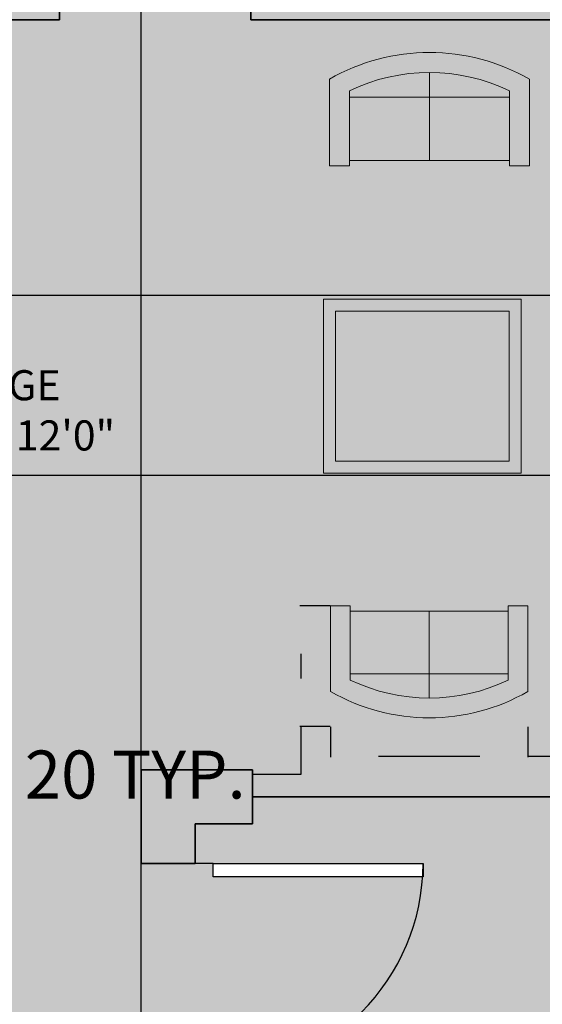
# Model space of a CAD drawing. Units: inches. Extents: x 389 to 971, y 148 to 870.
# Tile 12 of 14: x 670 to 757, y 428 to 592. Entities that reach past the tile are written whole.
import ezdxf

# ---------------------------------------------------------------- set-up
doc = ezdxf.new("R2010")
doc.units = ezdxf.units.IN
doc.header["$MEASUREMENT"] = 0
for name, color, linetype, lineweight in [('A-ANNO-DIMS', 2, 'Continuous', 18), ('A-AREA-IDEN', 7, 'Continuous', 18), ('A-DOOR', 4, 'Continuous', 25), ('A-FLOR-BASE-PATT', 8, 'Continuous', 13), ('A-FURN', 8, 'Continuous', 18), ('A-WALL', 7, 'Continuous', 35), ('L-GRND-BASE-PATT', 8, 'Continuous', 13)]:
    doc.layers.add(name, color=color, linetype=linetype, lineweight=lineweight)
for name, color, linetype, lineweight, true_color in [('A-FURN-SURF-PATT', 9, 'Continuous', 13, 0xd6bdce), ('A-WALL-PATT', 18, 'Continuous', 13, 0x000000), ('L-GRND-PATT', 39, 'Continuous', 13, 0x603913)]:
    doc.layers.add(name, color=color, linetype=linetype, lineweight=lineweight, true_color=true_color)
doc.styles.get("Standard").update_dxf_attribs({"font": 'arial.ttf'})
doc.dimstyles.get("Standard").update_dxf_attribs({"dimtxt": 8, "dimasz": 8, "dimexe": 0.18, "dimexo": 0.0625, "dimgap": 0.09, "dimtad": 0, "dimtih": 1, "dimtoh": 1, "dimdec": 0, "dimzin": 0, "dimdsep": 46, "dimlunit": 3, "dimtxsty": 'Standard', "dimcen": 0.09, "dimadec": 0, "dimazin": 0, "dimtfac": 1, "dimtdec": 0, "dimtofl": 0, "dimtmove": 0, "dimatfit": 3, "dimfxl": 1, "dimtolj": 1, "dimtzin": 0, "dimarcsym": 0})

# ---------------------------------------------------------------- blocks, each defined once
blk = doc.blocks.new('*U5')
for p, q in [((0, 0), (0, -6)), ((28, 0), (28, -6))]:
    blk.add_line(p, q)
blk.add_lwpolyline([(0, 0), (0, 28), (1.75, 28), (1.75, 0)], close=True)
blk.add_arc((0, 0), 28, 0, 90)
blk = doc.blocks.new('Sofa - Roundback Loveseat 5 ft.')
for p, q in [((0, -32.44198), (0, -5.99998)), ((-24, -33.99998), (-24, -11.46958)), ((24.00004, -33.99998), (24.00004, -11.46958)), ((-23.9998, -13.38178), (23.99986, -13.38178)), ((-24, -32.44198), (24.00004, -32.44198))]:
    blk.add_line(p, q)
for points in [[(-24, -33.99998), (-30, -33.99998), (-30, -7.99998)], [(30.00004, -7.99998), (30.00004, -33.99998), (24.00004, -33.99998)]]:
    blk.add_lwpolyline(points)
for centre, radius, start, end in [((0, -60.24998), 60.24998, 60.13715, 119.8628), ((0, -61.38438), 55.38444, 64.32083, 115.6792)]:
    blk.add_arc(centre, radius, start, end)
blk = doc.blocks.new('COFFEE-TABLE-RECT')
for points in [[(0, 28.98), (32.94, 28.98), (32.94, 0), (0, 0)], [(2, 26.98), (30.94, 26.98), (30.94, 2), (2, 2)]]:
    blk.add_lwpolyline(points, close=True)
blk = doc.blocks.new('*D40')
at = {"layer": 'A-ANNO-DIMS', "color": 0, "lineweight": -2, "transparency": 16777216}
for p, q in [((721.8, 473.76), (721.8, 468.71)), ((754.7, 473.76), (754.7, 468.71)), ((729.8, 468.89), (746.7, 468.89)), ((754.7, 468.89), (762.7, 468.89))]:
    blk.add_line(p, q, dxfattribs=at)
at = {"layer": 'A-ANNO-DIMS', "color": 0, "transparency": 16777216}
for points in [[(729.8, 470.23), (729.8, 467.56), (721.8, 468.89)], [(746.7, 470.23), (746.7, 467.56), (754.7, 468.89)]]:
    blk.add_solid(points, dxfattribs=at)
at = {"layer": 'Defpoints', "color": 0, "transparency": 16777216}
for p in [(721.8, 473.83), (754.7, 473.83), (754.7, 468.89)]:
    blk.add_point(p, dxfattribs=at)
at = {"layer": 'A-ANNO-DIMS', "color": 0, "transparency": 16777216, "insert": (813.14, 468.89), "char_height": 8, "attachment_point": 5}
blk.add_mtext('\\A1;LOVESEAT 33 TYP.', dxfattribs=at)
blk = doc.blocks.new('*D41')
at = {"layer": 'A-ANNO-DIMS', "color": 0, "lineweight": -2, "transparency": 16777216}
for p, q in [((721.74, 493.93), (716.69, 493.93)), ((716.87, 485.93), (716.87, 481.83)), ((721.74, 473.83), (716.69, 473.83)), ((716.87, 473.83), (716.87, 465.83)), ((716.87, 465.83), (708.87, 465.83))]:
    blk.add_line(p, q, dxfattribs=at)
at = {"layer": 'A-ANNO-DIMS', "color": 0, "transparency": 16777216}
for points in [[(715.53, 485.93), (718.2, 485.93), (716.87, 493.93)], [(715.53, 481.83), (718.2, 481.83), (716.87, 473.83)]]:
    blk.add_solid(points, dxfattribs=at)
at = {"layer": 'Defpoints', "color": 0, "transparency": 16777216}
for p in [(721.8, 493.93), (716.87, 473.83), (721.8, 473.83)]:
    blk.add_point(p, dxfattribs=at)
at = {"layer": 'A-ANNO-DIMS', "color": 0, "transparency": 16777216, "insert": (689.24, 465.83), "char_height": 8, "attachment_point": 5}
blk.add_mtext('\\A1;20 TYP.', dxfattribs=at)
blk = doc.blocks.new('*D48')
at = {"layer": 'A-ANNO-DIMS', "color": 0, "lineweight": -2, "transparency": 16777216}
for p, q in [((595.45, 545.73), (878.72, 545.73)), ((878.54, 537.73), (878.54, 534.91)), ((878.54, 523.73), (878.54, 526.55)), ((595.45, 515.73), (878.72, 515.73))]:
    blk.add_line(p, q, dxfattribs=at)
at = {"layer": 'A-ANNO-DIMS', "color": 0, "transparency": 16777216}
for points in [[(877.21, 537.73), (879.87, 537.73), (878.54, 545.73)], [(877.21, 523.73), (879.87, 523.73), (878.54, 515.73)]]:
    blk.add_solid(points, dxfattribs=at)
at = {"layer": 'Defpoints', "color": 0, "transparency": 16777216}
for p in [(595.39, 545.73), (878.54, 545.73), (595.39, 515.73)]:
    blk.add_point(p, dxfattribs=at)
at = {"layer": 'A-ANNO-DIMS', "color": 0, "transparency": 16777216, "insert": (878.54, 530.73), "char_height": 8, "attachment_point": 5}
blk.add_mtext('\\A1;30.005', dxfattribs=at)
blk = doc.blocks.new('*D52')
at = {"layer": 'A-ANNO-DIMS', "color": 0, "lineweight": -2, "transparency": 16777216}
for p, q in [((640.06, 864.97), (632.06, 864.97)), ((648.06, 388.98), (648.06, 865.15)), ((690.22, 388.98), (690.22, 865.15)), ((698.22, 864.97), (706.22, 864.97))]:
    blk.add_line(p, q, dxfattribs=at)
at = {"layer": 'A-ANNO-DIMS', "color": 0, "transparency": 16777216}
for points in [[(640.06, 866.3), (640.06, 863.64), (648.06, 864.97)], [(698.22, 866.3), (698.22, 863.64), (690.22, 864.97)]]:
    blk.add_solid(points, dxfattribs=at)
at = {"layer": 'Defpoints', "color": 0, "transparency": 16777216}
for p in [(690.22, 864.97), (648.06, 388.92), (690.22, 388.92)]:
    blk.add_point(p, dxfattribs=at)
at = {"layer": 'A-ANNO-DIMS', "color": 0, "transparency": 16777216, "insert": (669.14, 864.97), "char_height": 8, "attachment_point": 5}
blk.add_mtext('\\A1;42.155', dxfattribs=at)

msp = doc.modelspace()

# ---------------------------------------------------------------- hatches: boundary and pattern name
at = {"layer": 'A-FLOR-BASE-PATT'}
h = msp.add_hatch(color=256, dxfattribs=at)
h.dxf.hatch_style = 1
h.paths.add_polyline_path([(634.6594, 428.4021), (634.6594, 427.0792), (634.6305, 427.0792, -0.40145271), (604.4225, 398.1652), (604.0817, 398.1199, -0.40145271), (632.0195, 371.3788), (632.0462, 371.3788), (632.0462, 370.1554), (604.387, 370.1554), (604.387, 366.7191), (640.0296, 366.7191), (640.0296, 321.4969, 1), (647.061, 321.4969), (647.061, 412.9189), (690.216, 412.9189), (690.216, 416.0006), (694.716, 416.0006), (702.2145, 416.0006, 0.39601219), (737.1392, 448.8066), (702.2145, 448.8066), (702.2145, 450.9936), (694.716, 450.9936), (690.216, 450.9936), (690.216, 466.6012), (708.7881, 466.6012), (708.7881, 462.1012), (784.6145, 462.1012), (784.6145, 466.6012), (794.216, 466.6012), (794.216, 591.6445), (708.5171, 591.6445), (708.5171, 596.1445), (708.5171, 602.9755, 0.39601219), (678.6314, 634.7912), (678.6314, 602.9755), (676.6391, 602.9755), (676.6391, 596.1445), (676.6391, 591.6445), (661.216, 591.6445), (661.216, 632.6445), (653.109, 632.6445), (653.109, 641.6445), (653.109, 642.1751), (651.6417, 642.1751), (651.6417, 675.6801, 0.40145271), (619.5719, 642.1751), (619.5719, 637.1445), (619.5147, 632.6445), (604.387, 632.6445), (604.387, 545.7317), (595.3894, 545.7317), (595.3894, 544.4199), (565.4338, 544.4199, 0.40145271), (595.3894, 515.7475), (599.887, 515.7475), (604.387, 515.7271), (604.387, 428.4021)])
h.paths.add_polyline_path([(721.8003, 493.9292), (725.0899, 493.9292), (725.0899, 493.075), (751.4065, 493.075), (751.4065, 493.9292), (754.6961, 493.9292), (754.6961, 479.6744, -0.26666697), (721.8003, 479.6744)], flags=16)
h.paths.add_polyline_path([(720.6421, 516.0583), (720.6421, 545.0393), (753.5806, 545.0393), (753.5806, 516.0583)], flags=16)
h.paths.add_polyline_path([(722.6421, 518.0583), (722.6421, 543.0393), (751.5806, 543.0393), (751.5806, 518.0583)], flags=0)
h.paths.add_polyline_path([(763.7396, 488.5801), (763.7822, 488.1156), (764.1436, 488.1761)], flags=16)
h.paths.add_polyline_path([(777.9011, 479.7417), (778.0475, 480.1886), (777.4745, 480.275)], flags=16)
h.paths.add_polyline_path([(762.3329, 503.5919), (762.3329, 507.1718), (763.2624, 507.1718), (763.2624, 550.1306), (762.3329, 550.1306), (762.3329, 553.7105), (777.8458, 553.7105, -0.19047621), (777.8458, 503.5919)], flags=16)
h.paths.add_polyline_path([(721.6097, 567.2898), (721.6097, 581.7362, -0.26666697), (754.9475, 581.7362), (754.9475, 567.2898), (751.6137, 567.2898), (751.6137, 568.1555), (724.9435, 568.1555), (724.9435, 567.2898)], flags=16)
h.paths.add_polyline_path([(774.6347, 521.4914), (774.6347, 535.811), (778.6837, 535.811, -0.04962821), (778.6837, 521.4914)], flags=0)
h.paths.add_polyline_path([(764.6624, 576.8996), (764.7454, 576.4742), (765.0717, 576.4903)], flags=16)
h.paths.add_polyline_path([(777.2772, 570.3652), (777.4444, 570.8756), (776.7899, 570.9743)], flags=16)
h.paths.add_polyline_path([(644.2892, 516.9956), (685.2491, 516.9956), (685.2491, 535.7223), (644.2892, 535.7223)], flags=24)
h = msp.add_hatch(color=256, dxfattribs=at)
h.dxf.hatch_style = 1
h.paths.add_polyline_path([(699.216, 294.6445), (733.8057, 294.6445), (810.0514, 294.6445), (839.216, 294.6445), (839.216, 457.6012), (784.6145, 457.6012), (784.6145, 462.1012), (708.7881, 462.1012), (708.7881, 457.6012), (699.216, 457.6012), (699.216, 450.9936), (702.2145, 450.9936), (737.2076, 450.9936), (737.2076, 448.8066), (737.1392, 448.8066, -0.39601219), (702.2145, 416.0006), (699.216, 416.0006)])
h.paths.add_polyline_path([(755.1859, 373.9163), (788.1244, 373.9163), (788.1244, 344.9352), (755.1859, 344.9352)], flags=16)
h.paths.add_polyline_path([(757.1859, 371.9163), (786.1244, 371.9163), (786.1244, 346.9352), (757.1859, 346.9352)], flags=0)
h.paths.add_polyline_path([(746.1376, 327.3223), (750.14, 327.3223), (750.14, 326.2831), (798.1694, 326.2831), (798.1694, 327.3223), (802.1718, 327.3223), (802.1718, 309.9784, -0.19047621), (746.1376, 309.9784)], flags=16)
h.paths.add_polyline_path([(782.1596, 313.5685), (782.1596, 309.0415, -0.04962821), (766.1498, 309.0415), (766.1498, 313.5685)], flags=0)
h.paths.add_polyline_path([(804.6838, 390.5197), (803.6446, 390.5197), (803.6446, 394.5221), (820.9885, 394.5221, -0.19047621), (820.9885, 338.4879), (803.6446, 338.4879), (803.6446, 342.4903), (804.6838, 342.4903)], flags=16)
h.paths.add_polyline_path([(817.3984, 358.5001), (817.3984, 374.5099), (821.9254, 374.5099, -0.04962821), (821.9254, 358.5001)], flags=0)
h.paths.add_polyline_path([(806.8707, 326.6963), (806.4254, 327.1416), (806.4724, 326.6297)], flags=16)
h.paths.add_polyline_path([(822.0328, 317.4008), (822.1942, 317.8933), (821.5626, 317.9885)], flags=16)
h.paths.add_polyline_path([(808.1446, 418.9737), (808.2247, 418.5632), (808.5395, 418.5787)], flags=16)
h.paths.add_polyline_path([(820.3159, 412.669), (820.4772, 413.1615), (819.8457, 413.2568)], flags=16)
h.paths.add_polyline_path([(750.6082, 393.6667), (791.5681, 393.6667), (791.5681, 412.3933), (750.6082, 412.3933)], flags=24)
at = {"layer": 'A-FURN-SURF-PATT'}
h = msp.add_hatch(color=256, dxfattribs=at)
h.dxf.hatch_style = 1
h.paths.add_polyline_path([(754.9475, 581.7362, 0.26666697), (721.6097, 581.7362), (721.6097, 567.2898), (724.9435, 567.2898), (724.9435, 579.8081, -0.22792319), (751.6137, 579.8081), (751.6137, 567.2898), (754.9475, 567.2898)])
h = msp.add_hatch(color=256, dxfattribs=at)
h.dxf.hatch_style = 1
h.paths.add_polyline_path([(738.2786, 578.7459), (738.2786, 582.8475, 0.11251869), (724.9435, 579.8081), (724.9435, 578.7459)])
h = msp.add_hatch(color=256, dxfattribs=at)
h.dxf.hatch_style = 1
h.paths.add_polyline_path([(751.6137, 578.7459), (751.6137, 579.8081, 0.11251889), (738.2786, 582.8475), (738.2786, 578.7459)])
h = msp.add_hatch(color=256, dxfattribs=at)
h.dxf.hatch_style = 1
h.paths.add_polyline_path([(738.2786, 568.1555), (738.2786, 578.7459), (724.9435, 578.7459), (724.9435, 568.1555)])
h = msp.add_hatch(color=256, dxfattribs=at)
h.dxf.hatch_style = 1
h.paths.add_polyline_path([(751.6137, 568.1555), (751.6137, 578.7459), (738.2786, 578.7459), (738.2786, 568.1555)])
h = msp.add_hatch(color=256, dxfattribs=at)
h.dxf.hatch_style = 1
h.paths.add_polyline_path([(720.6421, 545.0393), (720.6421, 516.0583), (753.5806, 516.0583), (753.5806, 545.0393)])
h.paths.add_polyline_path([(751.5806, 543.0393), (751.5806, 518.0583), (722.6421, 518.0583), (722.6421, 543.0393)], flags=16)
h = msp.add_hatch(color=256, dxfattribs=at)
h.dxf.hatch_style = 1
h.paths.add_polyline_path([(751.5806, 518.0583), (751.5806, 543.0393), (722.6421, 543.0393), (722.6421, 518.0583)])
h = msp.add_hatch(color=256, dxfattribs=at)
h.dxf.hatch_style = 1
h.paths.add_polyline_path([(721.8003, 479.6744, 0.26666697), (754.6961, 479.6744), (754.6961, 493.9292), (751.4065, 493.9292), (751.4065, 481.5769, -0.22792319), (725.0899, 481.5769), (725.0899, 493.9292), (721.8003, 493.9292)])
h = msp.add_hatch(color=256, dxfattribs=at)
h.dxf.hatch_style = 1
h.paths.add_polyline_path([(738.2482, 493.075), (725.0899, 493.075), (725.0899, 482.625), (738.2482, 482.625)])
h = msp.add_hatch(color=256, dxfattribs=at)
h.dxf.hatch_style = 1
h.paths.add_polyline_path([(751.4065, 482.625), (751.4065, 493.075), (738.2482, 493.075), (738.2482, 482.625)])
h = msp.add_hatch(color=256, dxfattribs=at)
h.dxf.hatch_style = 1
h.paths.add_polyline_path([(738.2482, 482.625), (725.0899, 482.625), (725.0899, 481.5769, 0.11251869), (738.2482, 478.5778)])
h = msp.add_hatch(color=256, dxfattribs=at)
h.dxf.hatch_style = 1
h.paths.add_polyline_path([(751.4065, 481.5769), (751.4065, 482.625), (738.2482, 482.625), (738.2482, 478.5778, 0.11251889)])
at = {"layer": 'A-WALL-PATT'}
h = msp.add_hatch(color=256, dxfattribs=at)
h.dxf.hatch_style = 1
h.paths.add_polyline_path([(432.216, 434.6445), (436.3673, 434.6445), (436.3673, 443.6445), (432.216, 443.6445), (432.216, 830.6445), (746.216, 830.6445), (746.216, 823.8175), (755.216, 823.8175), (755.216, 825.6445), (839.216, 825.6445), (839.216, 803.5176), (839.216, 741.6445), (755.216, 741.6445), (755.216, 748.4596), (755.1859, 748.4596), (750.716, 748.4596), (746.216, 748.4596), (746.216, 732.6445), (839.216, 732.6445), (839.216, 600.6445), (708.5171, 600.6445), (708.5171, 596.1445), (708.5171, 591.6445), (794.216, 591.6445), (794.216, 587.4291), (803.216, 587.4291), (803.216, 591.6445), (839.216, 591.6445), (839.216, 466.6012), (803.216, 466.6012), (803.216, 471.0309), (794.216, 471.0309), (794.216, 466.6012), (784.6145, 466.6012), (784.6145, 457.6012), (839.216, 457.6012), (839.216, 447.6445), (839.216, 294.6445), (810.0514, 294.6445), (810.0514, 285.6445), (839.216, 285.6445), (839.216, 238.6445), (590.216, 238.6445), (590.216, 234.6445), (848.216, 234.6445), (848.216, 834.6445), (428.216, 834.6445), (428.216, 234.6445), (437.216, 234.6445), (437.216, 243.6445), (432.216, 243.6445)])
h = msp.add_hatch(color=256, dxfattribs=at)
h.dxf.hatch_style = 1
h.paths.add_polyline_path([(661.216, 785.6445), (661.216, 641.6445), (653.109, 641.6445), (653.109, 637.1445), (653.109, 632.6445), (661.216, 632.6445), (661.216, 591.6445), (676.6391, 591.6445), (676.6391, 600.6445), (670.216, 600.6445), (670.216, 785.6445), (685.2392, 785.6445), (685.2392, 794.6445), (662.4125, 794.6445), (606.2724, 794.6445), (606.2724, 785.6445), (616.7487, 785.6445)])
h = msp.add_hatch(color=256, dxfattribs=at)
h.dxf.hatch_style = 1
h.paths.add_polyline_path([(690.216, 466.6012), (690.216, 450.9936), (699.216, 450.9936), (699.216, 457.6012), (708.7881, 457.6012), (708.7881, 466.6012)])
at = {"layer": 'L-GRND-BASE-PATT'}
h = msp.add_hatch(color=256, dxfattribs=at)
h.dxf.hatch_style = 1
edge = h.paths.add_edge_path(flags=16)
edge.add_ellipse((8782.0026, 354.2473), major_axis=(-8296.9493, 0), ratio=0.84230387, start_angle=-0.09022909, end_angle=0.38386678, ccw=False)
edge.add_ellipse((485.0533, 368.2895), major_axis=(-1.1591, 0), ratio=0.84230387, start_angle=0, end_angle=90, ccw=False)
edge.add_line((483.8943, 368.2895), (483.8943, 387.6039))
edge.add_ellipse((485.0533, 387.2466), major_axis=(1.1591, 0), ratio=0.84230387, start_angle=90, end_angle=180, ccw=False)
edge.add_line((485.0533, 388.2229), (485.5047, 388.2229))
edge.add_ellipse((898.8202, 372.4897), major_axis=(413.7374, 0), ratio=0.84230387, start_angle=176.349572, end_angle=177.82005, ccw=False)
edge.add_ellipse((535.9119, 196.3855), major_axis=(-245.3972, 0), ratio=0.84230387, start_angle=-77.874034, end_angle=-76.219471, ccw=False)
edge.add_ellipse((535.9119, 201.7547), major_axis=(239.1274, 0), ratio=0.84230387, start_angle=100.209539, end_angle=102.444627, ccw=False)
edge.add_ellipse((473.3139, 564.9222), major_axis=(196.5637, 0), ratio=0.84230387, start_angle=-80.743434, end_angle=-77.445067)
edge.add_line((509.5535, 402.1941), (514.3535, 404.8483))
edge.add_line((514.3535, 404.8483), (514.3535, 404.7972))
edge.add_ellipse((514.3535, 404.2644), major_axis=(0.5795, 0), ratio=0.84230387, start_angle=52.06687, end_angle=90, ccw=False)
edge.add_line((514.6716, 404.6725), (519.1535, 402.1941))
edge.add_ellipse((555.3932, 564.9222), major_axis=(-196.5637, 0), ratio=0.84230387, start_angle=77.445067, end_angle=80.743434)
edge.add_ellipse((492.7951, 201.7547), major_axis=(239.1274, 0), ratio=0.84230387, start_angle=77.555373, end_angle=79.790461, ccw=False)
edge.add_ellipse((492.7951, 196.3855), major_axis=(245.3972, 0), ratio=0.84230387, start_angle=76.219471, end_angle=77.874034, ccw=False)
edge.add_ellipse((129.8868, 372.4897), major_axis=(-413.7374, 0), ratio=0.84230387, start_angle=182.17995, end_angle=183.650428, ccw=False)
edge.add_line((543.2023, 388.2229), (544.0779, 388.2229))
edge.add_ellipse((543.6537, 387.2466), major_axis=(-1.1591, 0), ratio=0.84230387, start_angle=180, end_angle=270, ccw=False)
edge.add_line((544.8128, 387.2466), (544.8128, 367.9322))
edge.add_ellipse((543.6537, 368.2895), major_axis=(1.1591, 0), ratio=0.84230387, start_angle=270, end_angle=360, ccw=False)
edge.add_ellipse((-7753.2956, 354.2473), major_axis=(-8296.9493, 0), ratio=0.84230387, start_angle=179.61613322, end_angle=180.09022909, ccw=False)
edge.add_line((543.3912, 298.6608), (544.0779, 298.6608))
edge.add_ellipse((543.6537, 297.6845), major_axis=(1.1591, 0), ratio=0.84230387, start_angle=0, end_angle=90, ccw=False)
edge.add_line((544.8128, 297.6845), (544.8128, 278.3701))
edge.add_ellipse((543.6537, 278.7275), major_axis=(-1.1591, 0), ratio=0.84230387, start_angle=90, end_angle=180, ccw=False)
edge.add_line((543.6537, 277.7512), (543.1566, 277.7512))
edge.add_ellipse((-7753.2956, 354.2473), major_axis=(-8296.9493, 0), ratio=0.84230387, start_angle=179.3813568, end_angle=179.47172853, ccw=False)
edge.add_ellipse((542.4236, 263.2763), major_axis=(-1.7386, 0), ratio=0.84230387, start_angle=179.371763, end_angle=248.464757, ccw=False)
edge.add_ellipse((-7753.8751, 354.2473), major_axis=(-8298.7403, 0), ratio=0.842303866, start_angle=179.35344592, end_angle=179.3717628, ccw=False)
edge.add_ellipse((540.0116, 260.6509), major_axis=(-4.1092, 0), ratio=0.84230387, start_angle=90, end_angle=179.353446, ccw=False)
edge.add_line((540.0116, 257.1897), (488.6954, 257.1897))
edge.add_ellipse((488.6954, 260.6509), major_axis=(4.1092, 0), ratio=0.84230387, start_angle=180.646554, end_angle=270, ccw=False)
edge.add_ellipse((8782.5821, 354.2473), major_axis=(-8298.7403, 0), ratio=0.842303872, start_angle=0.62823723, end_angle=0.64655411, ccw=False)
edge.add_ellipse((486.2834, 263.2763), major_axis=(-1.7386, 0), ratio=0.84230387, start_angle=-68.464756, end_angle=0.628237, ccw=False)
edge.add_ellipse((8782.0026, 354.2473), major_axis=(-8296.9493, 0), ratio=0.84230387, start_angle=0.52827147, end_angle=0.6465541, ccw=False)
edge.add_line((485.5504, 277.7512), (484.6291, 277.7512))
edge.add_ellipse((485.0533, 278.7275), major_axis=(-1.1591, 0), ratio=0.84230387, start_angle=0, end_angle=90, ccw=False)
edge.add_line((483.8943, 278.7275), (483.8943, 298.0418))
edge.add_ellipse((485.0533, 297.6845), major_axis=(1.1591, 0), ratio=0.84230387, start_angle=90, end_angle=180, ccw=False)
edge = h.paths.add_edge_path(flags=0)
edge.add_ellipse((8782.0026, 354.2473), major_axis=(-8295.7902, 0), ratio=0.84230387, start_angle=0.05559431, end_angle=0.37776419, ccw=False)
edge.add_line((486.2179, 346.1978), (489.3905, 335.8384))
edge.add_ellipse((3386.0114, 329.7263), major_axis=(-2896.63, 0), ratio=0.84230387, start_angle=-0.1208974, end_angle=0.3640763)
edge.add_line((489.4638, 311.3204), (486.4666, 299.5521))
edge = h.paths.add_edge_path(flags=0)
edge.add_ellipse((514.3535, 391.3731), major_axis=(-115.1513, 0), ratio=0.84230387, start_angle=76.401865, end_angle=103.598135)
edge.add_line((537.3428, 296.3333), (537.3428, 281.5897))
edge.add_ellipse((514.3535, 376.6295), major_axis=(-115.1513, 0), ratio=0.84230387, start_angle=76.401865, end_angle=103.598135, ccw=False)
edge.add_line((491.3643, 281.5897), (491.3643, 296.3333))
edge = h.paths.add_edge_path(flags=0)
edge.add_line((491.3643, 337.0752), (489.653, 349.9016))
edge.add_ellipse((510.1338, 298.7862), major_axis=(64.0481, 0), ratio=0.84230387, start_angle=94.277421, end_angle=111.834954, ccw=False)
edge.add_line((506.1068, 352.6274), (522.6002, 352.6274))
edge.add_ellipse((518.5732, 298.7862), major_axis=(64.0481, 0), ratio=0.84230387, start_angle=68.165046, end_angle=85.722579, ccw=False)
edge.add_line((539.0541, 349.9016), (537.3428, 337.0752))
edge.add_ellipse((516.5462, 287.5825), major_axis=(62.3305, 0), ratio=0.84230387, start_angle=67.208085, end_angle=85.12993)
edge.add_line((521.008, 339.949), (507.699, 339.949))
edge.add_ellipse((512.1609, 287.5825), major_axis=(62.3305, 0), ratio=0.84230387, start_angle=94.87007, end_angle=112.791915)
edge = h.paths.add_edge_path(flags=0)
edge.add_ellipse((493.6824, 273.9439), major_axis=(-2.3182, 0), ratio=0.84230387, start_angle=-90, end_angle=0, ccw=False)
edge.add_line((493.6824, 275.8965), (535.3743, 275.8965))
edge.add_ellipse((535.0246, 273.9439), major_axis=(2.3182, 0), ratio=0.84230387, start_angle=0, end_angle=90, ccw=False)
edge.add_line((537.3428, 273.9439), (537.3428, 258.6983))
edge.add_line((537.3428, 258.6983), (540.5912, 258.6983))
edge.add_ellipse((540.5912, 260.6509), major_axis=(-2.3182, 0), ratio=0.84230387, start_angle=90, end_angle=179.353446)
edge.add_line((540.5912, 258.6983), (487.7691, 258.6983))
edge.add_ellipse((488.1158, 260.6509), major_axis=(2.3182, 0), ratio=0.84230387, start_angle=180.646554, end_angle=270)
edge.add_line((488.1158, 258.6983), (491.3643, 258.6983))
edge.add_line((491.3643, 258.6983), (491.3643, 274.2384))
h.paths.add_polyline_path([(746.1376, 327.3223), (750.14, 327.3223), (750.14, 326.2831), (798.1694, 326.2831), (798.1694, 327.3223), (802.1718, 327.3223), (802.1718, 309.9784, -0.19047621), (746.1376, 309.9784)], flags=16)
h.paths.add_polyline_path([(782.1596, 313.5685), (782.1596, 309.0415, -0.04962821), (766.1498, 309.0415), (766.1498, 313.5685)], flags=0)
h.paths.add_polyline_path([(755.1859, 344.9352), (755.1859, 373.9163), (788.1244, 373.9163), (788.1244, 344.9352)], flags=16)
h.paths.add_polyline_path([(757.1859, 346.9352), (757.1859, 371.9163), (786.1244, 371.9163), (786.1244, 346.9352)], flags=0)
h.paths.add_polyline_path([(803.6446, 338.4879), (803.6446, 342.4903), (804.6838, 342.4903), (804.6838, 390.5197), (803.6446, 390.5197), (803.6446, 394.5221), (820.9885, 394.5221, -0.19047621), (820.9885, 338.4879)], flags=16)
h.paths.add_polyline_path([(806.8707, 326.6963), (806.4254, 327.1416), (806.4724, 326.6297)], flags=16)
h.paths.add_polyline_path([(822.0328, 317.4008), (822.1942, 317.8933), (821.5626, 317.9885)], flags=16)
h.paths.add_polyline_path([(817.3984, 358.5001), (817.3984, 374.5099), (821.9254, 374.5099, -0.04962821), (821.9254, 358.5001)], flags=0)
h.paths.add_polyline_path([(808.1446, 418.9737), (808.2247, 418.5632), (808.5395, 418.5787)], flags=16)
h.paths.add_polyline_path([(820.3159, 412.669), (820.4772, 413.1615), (819.8457, 413.2568)], flags=16)
h.paths.add_polyline_path([(466.3155, 235.5246), (517.3807, 235.5246), (517.3807, 244.4269), (466.3155, 244.4269)], flags=24)
h.paths.add_polyline_path([(739.8737, 256.2), (815.404, 256.2), (815.404, 265.3454), (739.8737, 265.3454)], flags=24)
h.paths.add_polyline_path([(750.6082, 393.6667), (791.5681, 393.6667), (791.5681, 412.3933), (750.6082, 412.3933)], flags=24)
h.paths.add_polyline_path([(438.9631, 410.0619), (484.6204, 410.0619), (484.6204, 429.1217), (438.9631, 429.1217)], flags=24)
edge = h.paths.add_edge_path()
edge.add_line((839.216, 285.6445), (611.8787, 285.6445))
edge.add_line((611.8787, 285.6445), (604.387, 285.6445))
edge.add_line((604.387, 285.6445), (595.387, 285.6445))
edge.add_line((595.387, 285.6445), (595.387, 370.1554))
edge.add_line((595.387, 370.1554), (604.0817, 370.1554))
edge.add_line((604.0817, 370.1554), (604.0817, 371.3788))
edge.add_line((604.0817, 371.3788), (632.0195, 371.3788))
edge.add_arc((604.0817, 370.1554), 27.9645, 2.507491, 90)
edge.add_line((604.0817, 398.1199), (599.887, 398.1652))
edge.add_line((599.887, 398.1652), (604.4225, 398.1652))
edge.add_arc((604.4225, 428.4021), 30.2369, 270, 357.492509)
edge.add_line((634.6305, 427.0792), (604.4225, 427.0792))
edge.add_line((604.4225, 427.0792), (604.4225, 428.4021))
edge.add_line((604.4225, 428.4021), (599.887, 428.4021))
edge.add_line((599.887, 428.4021), (595.387, 428.4021))
edge.add_line((595.387, 428.4021), (595.387, 434.6445))
edge.add_line((595.387, 434.6445), (585.0791, 434.6445))
edge.add_line((585.0791, 434.6445), (540.3922, 434.6445))
edge.add_line((540.3922, 434.6445), (526.7125, 434.6445))
edge.add_line((526.7125, 434.6445), (488.4095, 434.6445))
edge.add_line((488.4095, 434.6445), (432.216, 434.6445))
edge.add_line((432.216, 434.6445), (432.216, 243.6445))
edge.add_line((432.216, 243.6445), (437.216, 243.6445))
edge.add_line((437.216, 243.6445), (437.216, 234.6445))
edge.add_line((437.216, 234.6445), (581.216, 234.6445))
edge.add_line((581.216, 234.6445), (581.216, 238.6445))
edge.add_line((581.216, 238.6445), (581.216, 243.6445))
edge.add_line((581.216, 243.6445), (590.216, 243.6445))
edge.add_line((590.216, 243.6445), (590.216, 238.6445))
edge.add_line((590.216, 238.6445), (839.216, 238.6445))
edge.add_line((839.216, 238.6445), (839.216, 285.6445))
at = {"layer": 'L-GRND-PATT'}
h = msp.add_hatch(dxfattribs=at)
h.set_pattern_fill('EARTH', color=256, angle=45)
h.set_pattern_definition([(45, (0, 0), (0, 8.980256), [6.35, -6.35]), (45, (-1.684, 1.684), (0, 8.980256), [6.35, -6.35]), (45, (-3.3676, 3.3676), (0, 8.980256), [6.35, -6.35]), (135, (-3.3676, 4.49), (-8.980256, 0), [6.35, -6.35]), (135, (-1.684, 6.174), (-8.980256, 0), [6.35, -6.35]), (135, (0, 7.858), (-8.980256, 0), [6.35, -6.35])])
h.paths.add_polyline_path([(432.216, 243.6445), (437.216, 243.6445), (437.216, 234.6445), (581.216, 234.6445), (581.216, 238.6445), (581.216, 243.6445), (590.216, 243.6445), (590.216, 238.6445), (839.216, 238.6445), (839.216, 285.6445), (810.0514, 285.6445), (733.8057, 285.6445), (684.2434, 285.6445), (611.8787, 285.6445), (604.387, 285.6445), (595.387, 285.6445), (595.387, 370.1554), (604.0817, 370.1554), (604.0817, 371.3788), (632.0195, 371.3788, 0.40145271), (604.0817, 398.1199), (599.887, 398.1652), (604.4225, 398.1652, 0.40145271), (634.6305, 427.0792), (604.4225, 427.0792), (604.4225, 428.4021), (599.887, 428.4021), (595.387, 428.4021), (595.387, 434.6445), (585.0791, 434.6445), (540.3922, 434.6445), (526.7125, 434.6445), (488.4095, 434.6445), (432.216, 434.6445)])
edge = h.paths.add_edge_path(flags=16)
edge.add_line((483.8943, 278.7275), (483.8943, 298.2564))
edge.add_ellipse((485.0533, 297.6845), major_axis=(1.1591, 0), ratio=0.84230387, start_angle=90, end_angle=180, ccw=False)
edge.add_ellipse((8782.0026, 354.2473), major_axis=(-8296.9493, 0), ratio=0.84230387, start_angle=-0.09022909, end_angle=0.38386678, ccw=False)
edge.add_ellipse((485.0533, 368.2895), major_axis=(-1.1591, 0), ratio=0.84230387, start_angle=0, end_angle=90, ccw=False)
edge.add_line((483.8943, 368.2895), (483.8943, 387.8185))
edge.add_ellipse((485.0533, 387.2466), major_axis=(1.1591, 0), ratio=0.84230387, start_angle=90, end_angle=180, ccw=False)
edge.add_ellipse((898.8202, 372.4897), major_axis=(413.7374, 0), ratio=0.84230387, start_angle=176.349572, end_angle=177.82005, ccw=False)
edge.add_ellipse((535.9119, 196.3855), major_axis=(-245.3972, 0), ratio=0.84230387, start_angle=-77.874034, end_angle=-76.219471, ccw=False)
edge.add_ellipse((535.9119, 201.7547), major_axis=(239.1274, 0), ratio=0.84230387, start_angle=100.209539, end_angle=102.444627, ccw=False)
edge.add_ellipse((473.3139, 564.9222), major_axis=(196.5637, 0), ratio=0.84230387, start_angle=-80.743434, end_angle=-77.445067)
edge.add_line((509.5535, 402.1941), (514.3535, 404.8483))
edge.add_line((514.3535, 404.8483), (519.1535, 402.1941))
edge.add_ellipse((555.3932, 564.9222), major_axis=(-196.5637, 0), ratio=0.84230387, start_angle=77.445067, end_angle=80.743434)
edge.add_ellipse((492.7951, 201.7547), major_axis=(239.1274, 0), ratio=0.84230387, start_angle=77.555373, end_angle=79.790461, ccw=False)
edge.add_ellipse((492.7951, 196.3855), major_axis=(245.3972, 0), ratio=0.84230387, start_angle=76.219471, end_angle=77.874034, ccw=False)
edge.add_ellipse((129.8868, 372.4897), major_axis=(-413.7374, 0), ratio=0.84230387, start_angle=182.17995, end_angle=183.650428, ccw=False)
edge.add_line((543.2023, 388.2229), (544.3327, 388.2229))
edge.add_ellipse((543.6537, 387.2466), major_axis=(-1.1591, 0), ratio=0.84230387, start_angle=180, end_angle=270, ccw=False)
edge.add_line((544.8128, 387.2466), (544.8128, 367.7176))
edge.add_ellipse((543.6537, 368.2895), major_axis=(1.1591, 0), ratio=0.84230387, start_angle=270, end_angle=360, ccw=False)
edge.add_ellipse((-7753.2956, 354.2473), major_axis=(-8296.9493, 0), ratio=0.84230387, start_angle=179.61613322, end_angle=180.09022909, ccw=False)
edge.add_ellipse((543.6537, 297.6845), major_axis=(1.1591, 0), ratio=0.84230387, start_angle=0, end_angle=90, ccw=False)
edge.add_line((544.8128, 297.6845), (544.8128, 278.1556))
edge.add_ellipse((543.6537, 278.7275), major_axis=(-1.1591, 0), ratio=0.84230387, start_angle=90, end_angle=180, ccw=False)
edge.add_ellipse((-7753.2956, 354.2473), major_axis=(-8296.9493, 0), ratio=0.84230387, start_angle=179.3813568, end_angle=179.47172853, ccw=False)
edge.add_ellipse((542.4236, 263.2763), major_axis=(-1.7386, 0), ratio=0.84230387, start_angle=179.371763, end_angle=248.464757, ccw=False)
edge.add_ellipse((-7753.8751, 354.2473), major_axis=(-8298.7403, 0), ratio=0.842303866, start_angle=179.35344592, end_angle=179.3717628, ccw=False)
edge.add_ellipse((540.0116, 260.6509), major_axis=(-4.1092, 0), ratio=0.84230387, start_angle=90, end_angle=179.353446, ccw=False)
edge.add_line((540.0116, 257.1897), (488.0808, 257.1897))
edge.add_ellipse((488.6954, 260.6509), major_axis=(4.1092, 0), ratio=0.84230387, start_angle=180.646554, end_angle=270, ccw=False)
edge.add_ellipse((8782.5821, 354.2473), major_axis=(-8298.7403, 0), ratio=0.842303872, start_angle=0.62823723, end_angle=0.64655411, ccw=False)
edge.add_ellipse((486.2834, 263.2763), major_axis=(-1.7386, 0), ratio=0.84230387, start_angle=-68.464756, end_angle=0.628237, ccw=False)
edge.add_ellipse((8782.0026, 354.2473), major_axis=(-8296.9493, 0), ratio=0.84230387, start_angle=0.52827147, end_angle=0.6465541, ccw=False)
edge.add_line((485.5504, 277.7512), (484.3744, 277.7512))
edge.add_ellipse((485.0533, 278.7275), major_axis=(-1.1591, 0), ratio=0.84230387, start_angle=0, end_angle=90, ccw=False)
edge = h.paths.add_edge_path(flags=0)
edge.add_ellipse((488.1158, 260.6509), major_axis=(2.3182, 0), ratio=0.84230387, start_angle=180.646554, end_angle=270)
edge.add_line((488.1158, 258.6983), (491.3643, 258.6983))
edge.add_line((491.3643, 258.6983), (491.3643, 274.4686))
edge.add_ellipse((493.6824, 273.9439), major_axis=(-2.3182, 0), ratio=0.84230387, start_angle=-90, end_angle=0, ccw=False)
edge.add_line((493.6824, 275.8965), (535.6476, 275.8965))
edge.add_ellipse((535.0246, 273.9439), major_axis=(2.3182, 0), ratio=0.84230387, start_angle=0, end_angle=90, ccw=False)
edge.add_line((537.3428, 273.9439), (537.3428, 258.6983))
edge.add_line((537.3428, 258.6983), (541.2086, 258.6983))
edge.add_ellipse((540.5912, 260.6509), major_axis=(-2.3182, 0), ratio=0.84230387, start_angle=90, end_angle=179.353446, ccw=False)
edge.add_line((540.5912, 258.6983), (487.4984, 258.6983))
edge = h.paths.add_edge_path(flags=0)
edge.add_line((491.3643, 281.5897), (491.3643, 296.3333))
edge.add_ellipse((514.3535, 391.3731), major_axis=(-115.1513, 0), ratio=0.84230387, start_angle=76.401865, end_angle=103.598135)
edge.add_line((537.3428, 296.3333), (537.3428, 281.5897))
edge.add_ellipse((514.3535, 376.6295), major_axis=(-115.1513, 0), ratio=0.84230387, start_angle=76.401865, end_angle=103.598135, ccw=False)
edge = h.paths.add_edge_path(flags=0)
edge.add_ellipse((8782.0026, 354.2473), major_axis=(-8295.7902, 0), ratio=0.84230387, start_angle=0.05559431, end_angle=0.37776419, ccw=False)
edge.add_line((486.2179, 346.1978), (489.3905, 335.8384))
edge.add_ellipse((3386.0114, 329.7263), major_axis=(-2896.63, 0), ratio=0.84230387, start_angle=-0.1208974, end_angle=0.3640763)
edge.add_line((489.4638, 311.3204), (486.4666, 299.5521))
edge = h.paths.add_edge_path(flags=0)
edge.add_line((491.3643, 337.0752), (489.653, 349.9016))
edge.add_ellipse((510.1338, 298.7862), major_axis=(64.0481, 0), ratio=0.84230387, start_angle=94.277421, end_angle=111.834954, ccw=False)
edge.add_line((506.1068, 352.6274), (522.6002, 352.6274))
edge.add_ellipse((518.5732, 298.7862), major_axis=(64.0481, 0), ratio=0.84230387, start_angle=68.165046, end_angle=85.722579, ccw=False)
edge.add_line((539.0541, 349.9016), (537.3428, 337.0752))
edge.add_ellipse((516.5462, 287.5825), major_axis=(62.3305, 0), ratio=0.84230387, start_angle=67.208085, end_angle=85.12993)
edge.add_line((521.008, 339.949), (507.699, 339.949))
edge.add_ellipse((512.1609, 287.5825), major_axis=(62.3305, 0), ratio=0.84230387, start_angle=94.87007, end_angle=112.791915)
h.paths.add_polyline_path([(466.3155, 235.5246), (517.3807, 235.5246), (517.3807, 244.4269), (466.3155, 244.4269)], flags=24)
h.paths.add_polyline_path([(739.8737, 256.2), (815.404, 256.2), (815.404, 265.3454), (739.8737, 265.3454)], flags=24)
h.paths.add_polyline_path([(438.9631, 410.0619), (484.6204, 410.0619), (484.6204, 429.1217), (438.9631, 429.1217)], flags=24)

# ---------------------------------------------------------------- linework, layer by layer
at = {"layer": 'A-WALL'}
for p, q in [((676.6391, 600.6445), (676.6391, 591.6445)), ((708.5171, 596.1445), (708.5171, 591.6445)), ((676.6391, 591.6445), (661.216, 591.6445)), ((794.216, 591.6445), (708.5171, 591.6445)), ((794.216, 591.6445), (746.216, 591.6445)), ((708.7881, 466.6012), (690.216, 466.6012)), ((690.216, 450.9936), (690.216, 466.6012)), ((708.7881, 466.6012), (708.7881, 457.6012)), ((784.6145, 462.1012), (708.7881, 462.1012)), ((708.7881, 457.6012), (699.216, 457.6012)), ((699.216, 450.9936), (699.216, 457.6012)), ((690.216, 450.9936), (699.216, 450.9936))]:
    msp.add_line(p, q, dxfattribs=at)

# ---------------------------------------------------------------- block references
at = {"layer": 'A-DOOR', "xscale": 1.249752530320971, "yscale": 1.249752530320971, "zscale": 1.249752530320971, "rotation": 270}
msp.add_blockref('*U5', (702.2145, 450.9936), dxfattribs=at)
at = {"layer": 'A-FURN', "xscale": 0.555629709431333, "yscale": 0.555629709431333, "zscale": 0.555629709431333}
msp.add_blockref('Sofa - Roundback Loveseat 5 ft.', (738.2786, 586.1812), dxfattribs=at)
at = {"layer": 'A-FURN'}
msp.add_blockref('COFFEE-TABLE-RECT', (720.6421, 516.0583), dxfattribs=at)
at = {"layer": 'A-FURN', "xscale": -0.5482635908218306, "yscale": 0.5482635908218306, "zscale": 0.5482635908218306, "rotation": 180}
msp.add_blockref('Sofa - Roundback Loveseat 5 ft.', (738.2482, 475.2883), dxfattribs=at)

# ---------------------------------------------------------------- texts
at = {"layer": 'A-AREA-IDEN', "insert": (646.3073, 533.2284), "char_height": 5.018573, "attachment_point": 1}
msp.add_mtext_dynamic_manual_height_columns('  LOUNGE\\P15\'7" x 12\'0"', width=113.900213, gutter_width=25.0929, heights=[0], dxfattribs=at)

# ---------------------------------------------------------------- dimensions: what is measured, and where the dimension line sits
at = {"layer": 'A-ANNO-DIMS'}
dim = msp.add_linear_dim(base=(690.216, 864.9695), p1=(648.061, 388.9189), p2=(690.216, 388.9189), dimstyle='Standard', override={"dimdec": 3, "dimlfac": 1, "dimrnd": 0, "dimzin": 0, "dimdsep": 46, "dimlunit": 2}, dxfattribs=at)
dim.commit()
dim.dimension.update_dxf_attribs({"geometry": '*D52', "text_midpoint": (669.1385, 864.9695)})
dim = msp.add_linear_dim(base=(878.541, 545.7317), p1=(595.387, 515.7271), p2=(595.387, 545.7317), angle=90, dimstyle='Standard', override={"dimdec": 3, "dimlfac": 1, "dimrnd": 0, "dimzin": 0, "dimdsep": 46, "dimlunit": 2}, dxfattribs=at)
dim.commit()
dim.dimension.update_dxf_attribs({"geometry": '*D48', "text_midpoint": (878.541, 530.7294)})
dim = msp.add_linear_dim(base=(716.8659, 473.8262), p1=(721.8003, 493.9292), p2=(721.8003, 473.8262), angle=270, text='<> TYP.', dimstyle='Standard', override={"dimdec": 0, "dimlfac": 1, "dimrnd": 0, "dimzin": 0, "dimdsep": 46, "dimlunit": 2}, dxfattribs=at)
dim.commit()
dim.dimension.update_dxf_attribs({"geometry": '*D41', "text_midpoint": (689.237, 465.8262)})
dim = msp.add_linear_dim(base=(754.6961, 468.8918), p1=(721.8003, 473.8262), p2=(754.6961, 473.8262), text='LOVESEAT <> TYP.', dimstyle='Standard', override={"dimdec": 0, "dimlfac": 1, "dimrnd": 0, "dimzin": 0, "dimdsep": 46, "dimlunit": 2}, dxfattribs=at)
dim.commit()
dim.dimension.update_dxf_attribs({"geometry": '*D40', "text_midpoint": (813.1354, 468.8918)})

doc.saveas('drawing.dxf')
